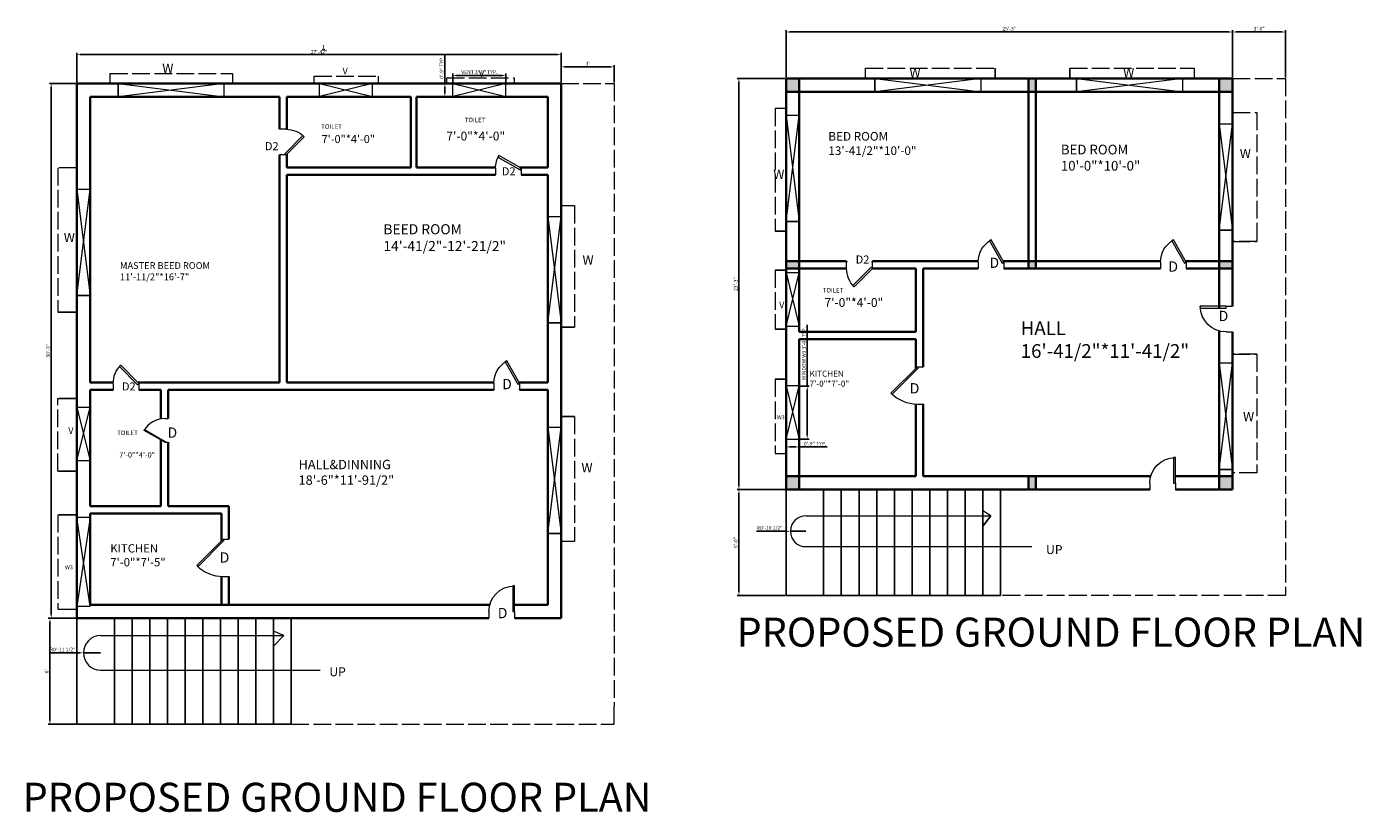
# Model space of a CAD drawing. Units: millimetres. Extents: x 3312 to 4717, y 967 to 1587.
# Tile 2 of 2: x 3811 to 4717, y 1054 to 1587. Entities that reach past the tile are written whole.
import ezdxf

# ---------------------------------------------------------------- set-up
doc = ezdxf.new("R2010")
doc.units = ezdxf.units.MM
doc.linetypes.add('ACAD_ISO02W100', pattern=[15, 12, -3])
for name, color, linetype, lineweight, true_color in [('A-ANNO-DIMS', 116, 'Continuous', 18, 0x136734), ('A-ANNO-IDEN', 116, 'Continuous', 18, 0x136734), ('A-ANNO-SYMB', 219, 'Continuous', 18, 0x642165), ('A-ANNO-TEXT', 55, 'Continuous', 18, 0x999b37), ('A-ANNO-TITL', 116, 'Continuous', 35, 0x136734), ('A-AREA-IDEN', 244, 'Continuous', 18, 0x991b1e), ('A-GLAZ', 219, 'Continuous', 18, 0x642165), ('A-GLAZ-OVHD', 67, 'ACAD_ISO02W100', 13, 0x727430), ('C-PROP', 67, 'ACAD_ISO02W100', 18, 0x727430)]:
    doc.layers.add(name, color=color, linetype=linetype, lineweight=lineweight, true_color=true_color)
for name, color, linetype, lineweight in [('A-COLS', 7, 'Continuous', 35), ('A-COLS-PATT', 7, 'Continuous', 13), ('A-DOOR', 4, 'Continuous', 18), ('A-FLOR-STRS', 7, 'Continuous', 25), ('A-WALL', 7, 'Continuous', 35)]:
    doc.layers.add(name, color=color, linetype=linetype, lineweight=lineweight)
doc.styles.get("Standard").update_dxf_attribs({"font": 'arial.ttf'})
doc.dimstyles.new('ISO-25', dxfattribs={"dimtxt": 2.5, "dimasz": 2.5, "dimexe": 1.25, "dimexo": 0.625, "dimtad": 1, "dimdec": 3, "dimlunit": 4, "dimtxsty": 'Standard', "dimcen": 2.5, "dimadec": 0, "dimazin": 0, "dimtfac": 1, "dimtdec": 3, "dimtmove": 0, "dimatfit": 3, "dimfxl": 1, "dimarcsym": 0})

# ---------------------------------------------------------------- blocks, each defined once
blk = doc.blocks.new('*U2')
for p, q in [((0, 0), (0, -6)), ((24, 0), (24, -6))]:
    blk.add_line(p, q)
blk.add_lwpolyline([(0, 0), (0, 24), (1.75, 24), (1.75, 0)], close=True)
blk.add_arc((0, 0), 24, 0, 90)
blk = doc.blocks.new('*U13')
for p, q in [((0, 0), (0, -6)), ((24, 0), (24, -6))]:
    blk.add_line(p, q)
blk.add_lwpolyline([(0, 0), (12, 20.8), (13.5, 19.9), (1.5, -0.9)], close=True)
blk.add_arc((0, 0), 24, 0, 60)
blk = doc.blocks.new('*U15')
for p, q in [((0, 0), (0, -6)), ((24, 0), (24, -6))]:
    blk.add_line(p, q)
blk.add_lwpolyline([(0, 0), (20.8, 12), (21.7, 10.5), (0.9, -1.5)], close=True)
blk.add_arc((0, 0), 24, 0, 30)
blk = doc.blocks.new('*U6')
for p, q in [((0, 0), (0, 6)), ((40, 0), (40, 6))]:
    blk.add_line(p, q)
blk.add_lwpolyline([(0, 0), (28.3, -28.3), (29.5, -27), (1.2, 1.2)], close=True)
blk.add_arc((0, 0), 40, 315, 360)
blk = doc.blocks.new('*U14')
for p, q in [((0, 0), (0, -6)), ((24, 0), (24, -6))]:
    blk.add_line(p, q)
blk.add_lwpolyline([(0, 0), (17, 17), (18.2, 15.7), (1.2, -1.2)], close=True)
blk.add_arc((0, 0), 24, 0, 45)
blk = doc.blocks.new('*U7')
for p, q in [((0, 0), (0, -6)), ((40, 0), (40, -6))]:
    blk.add_line(p, q)
blk.add_lwpolyline([(0, 0), (20, 34.6), (21.5, 33.8), (1.5, -0.9)], close=True)
blk.add_arc((0, 0), 40, 0, 60)
blk = doc.blocks.new('*D16')
at = {"layer": 'A-ANNO-DIMS', "color": 0, "lineweight": -2, "transparency": 16777216}
for p, q in [((4174.05, 1549.21), (4174.05, 1561.11)), ((4176.55, 1559.86), (4207.55, 1559.86)), ((4210.05, 1549.21), (4210.05, 1561.11))]:
    blk.add_line(p, q, dxfattribs=at)
at = {"layer": 'A-ANNO-DIMS', "color": 0, "lineweight": 5, "transparency": 16777216}
for points in [[(4176.55, 1560.28), (4176.55, 1559.45), (4174.05, 1559.86)], [(4207.55, 1560.28), (4207.55, 1559.45), (4210.05, 1559.86)]]:
    blk.add_solid(points, dxfattribs=at)
at = {"layer": 'Defpoints', "color": 0, "lineweight": 5, "transparency": 16777216}
for p in [(4210.05, 1559.86), (4174.05, 1548.59), (4210.05, 1548.59)]:
    blk.add_point(p, dxfattribs=at)
at = {"layer": 'A-ANNO-DIMS', "color": 0, "transparency": 16777216, "insert": (4192.05, 1561.76), "char_height": 2.5, "attachment_point": 5}
blk.add_mtext("3'", dxfattribs=at)
blk = doc.blocks.new('*D17')
at = {"layer": 'A-ANNO-DIMS', "color": 0, "lineweight": -2, "transparency": 16777216}
for p, q in [((3845.55, 1549.21), (3845.55, 1569.4)), ((4171.55, 1568.15), (3848.05, 1568.15)), ((4174.05, 1549.21), (4174.05, 1569.4))]:
    blk.add_line(p, q, dxfattribs=at)
at = {"layer": 'A-ANNO-DIMS', "color": 0, "lineweight": 5, "transparency": 16777216}
for points in [[(3848.05, 1568.56), (3848.05, 1567.73), (3845.55, 1568.15)], [(4171.55, 1568.56), (4171.55, 1567.73), (4174.05, 1568.15)]]:
    blk.add_solid(points, dxfattribs=at)
at = {"layer": 'Defpoints', "color": 0, "lineweight": 5, "transparency": 16777216}
for p in [(3845.55, 1568.15), (3845.55, 1548.59), (4174.05, 1548.59)]:
    blk.add_point(p, dxfattribs=at)
at = {"layer": 'A-ANNO-DIMS', "color": 0, "transparency": 16777216, "insert": (4009.8, 1571.7), "char_height": 2.5, "attachment_point": 5}
blk.add_mtext('27\'-4{\\H1x;\\S1/2;}"', dxfattribs=at)
blk = doc.blocks.new('*D18')
at = {"layer": 'A-ANNO-DIMS', "color": 0, "lineweight": -2, "transparency": 16777216}
for p, q in [((3844.92, 1548.59), (3826.85, 1548.59)), ((3828.1, 1546.09), (3828.1, 1188.09)), ((3844.92, 1185.59), (3826.85, 1185.59))]:
    blk.add_line(p, q, dxfattribs=at)
at = {"layer": 'A-ANNO-DIMS', "color": 0, "lineweight": 5, "transparency": 16777216}
for points in [[(3827.69, 1546.09), (3828.52, 1546.09), (3828.1, 1548.59)], [(3827.69, 1188.09), (3828.52, 1188.09), (3828.1, 1185.59)]]:
    blk.add_solid(points, dxfattribs=at)
at = {"layer": 'Defpoints', "color": 0, "lineweight": 5, "transparency": 16777216}
for p in [(3845.55, 1548.59), (3828.1, 1185.59), (3845.55, 1185.59)]:
    blk.add_point(p, dxfattribs=at)
at = {"layer": 'A-ANNO-DIMS', "color": 0, "transparency": 16777216, "insert": (3826.2, 1367.09), "char_height": 2.5, "attachment_point": 5, "rotation": 90}
blk.add_mtext('30\'-3"', dxfattribs=at)
blk = doc.blocks.new('*D19')
at = {"layer": 'A-ANNO-DIMS', "color": 0, "lineweight": -2, "transparency": 16777216}
for p, q in [((3844.92, 1185.59), (3825.98, 1185.59)), ((3827.23, 1183.09), (3827.23, 1116.09)), ((3844.92, 1113.59), (3825.98, 1113.59))]:
    blk.add_line(p, q, dxfattribs=at)
at = {"layer": 'A-ANNO-DIMS', "color": 0, "lineweight": 5, "transparency": 16777216}
for points in [[(3826.82, 1183.09), (3827.65, 1183.09), (3827.23, 1185.59)], [(3826.82, 1116.09), (3827.65, 1116.09), (3827.23, 1113.59)]]:
    blk.add_solid(points, dxfattribs=at)
at = {"layer": 'Defpoints', "color": 0, "lineweight": 5, "transparency": 16777216}
for p in [(3845.55, 1185.59), (3827.23, 1113.59), (3845.55, 1113.59)]:
    blk.add_point(p, dxfattribs=at)
at = {"layer": 'A-ANNO-DIMS', "color": 0, "transparency": 16777216, "insert": (3825.33, 1149.59), "char_height": 2.5, "attachment_point": 5, "rotation": 90}
blk.add_mtext("6'", dxfattribs=at)
blk = doc.blocks.new('*U21')
for p, q in [((0, 0), (0, -6)), ((24, 0), (24, -6))]:
    blk.add_line(p, q)
blk.add_lwpolyline([(0, 0), (0, 24), (1.75, 24), (1.75, 0)], close=True)
blk.add_arc((0, 0), 24, 0, 90)
blk = doc.blocks.new('*U20')
for p, q in [((0, 0), (0, 6)), ((24, 0), (24, 6))]:
    blk.add_line(p, q)
blk.add_lwpolyline([(0, 0), (17, -17), (18.2, -15.7), (1.2, 1.2)], close=True)
blk.add_arc((0, 0), 24, 315, 0)
blk = doc.blocks.new('WIN-STANDARD')
for p, q in [((0, 72), (0, 0)), ((0, 0), (9, 72)), ((9, 72), (0, 72)), ((0, 72), (9, 0)), ((9, 0), (9, 72)), ((0, 0), (9, 0)), ((9, 0), (0, 0))]:
    blk.add_line(p, q)
blk = doc.blocks.new('GLAZ-NARROW')
for p, q in [((9, 35.99), (0.01, 35.99)), ((0.01, 35.99), (0.01, 0)), ((0.01, 0), (9, 35.99)), ((0.07, 35.99), (9, 0)), ((9, 0), (9, 35.99)), ((0, 0), (9, 0))]:
    blk.add_line(p, q)
blk = doc.blocks.new('VENT-PLAN')
for p, q in [((36, 9.18), (0, 9.18)), ((36, 9.18), (0, 0.18)), ((0, 0.18), (0, 9.18)), ((0, 9.18), (36, 0.18)), ((36, 0), (36, 9.18)), ((0, 0.18), (36, 0.18))]:
    blk.add_line(p, q)
blk = doc.blocks.new('STAIR-ENTRY-FLIGHT')
for p, q in [((0, 72), (0, 0)), ((145.5, 72), (0, 72)), ((25.5, 0), (25.5, 72)), ((37.5, 0), (37.5, 72)), ((49.5, 0), (49.5, 72)), ((61.5, 0), (61.5, 72)), ((73.5, 0), (73.5, 72)), ((85.5, 0), (85.5, 72)), ((97.5, 0), (97.5, 72)), ((109.5, 0), (109.5, 72)), ((121.5, 0), (121.5, 72)), ((133.5, 0), (133.5, 72)), ((145.5, 0), (145.5, 72)), ((0, 0), (145.5, 0))]:
    blk.add_line(p, q)
blk = doc.blocks.new('*D28')
at = {"layer": 'A-ANNO-DIMS', "color": 0, "lineweight": -2, "transparency": 16777216}
for p, q in [((4341.03, 1343.2), (4341.03, 1384.8)), ((4336.26, 1343.2), (4342.28, 1343.2)), ((4341.03, 1309.72), (4341.03, 1340.7)), ((4336.26, 1307.22), (4342.28, 1307.22))]:
    blk.add_line(p, q, dxfattribs=at)
at = {"layer": 'A-ANNO-DIMS', "color": 0, "lineweight": 5, "transparency": 16777216}
for points in [[(4340.61, 1340.7), (4341.45, 1340.7), (4341.03, 1343.2)], [(4340.61, 1309.72), (4341.45, 1309.72), (4341.03, 1307.22)]]:
    blk.add_solid(points, dxfattribs=at)
at = {"layer": 'Defpoints', "color": 0, "lineweight": 5, "transparency": 16777216}
for p in [(4335.63, 1343.2), (4341.03, 1343.2), (4335.63, 1307.22)]:
    blk.add_point(p, dxfattribs=at)
at = {"layer": 'A-ANNO-DIMS', "color": 0, "transparency": 16777216, "insert": (4339.11, 1365.25), "char_height": 2.5, "attachment_point": 5, "rotation": 90}
blk.add_mtext('WINDOW W3 3\'-0" TYP.', dxfattribs=at)
blk = doc.blocks.new('*D29')
at = {"layer": 'A-ANNO-DIMS', "color": 0, "lineweight": -2, "transparency": 16777216}
for p, q in [((4326.63, 1306.59), (4326.63, 1300.57)), ((4335.63, 1306.59), (4335.63, 1300.57)), ((4329.13, 1301.82), (4333.13, 1301.82)), ((4335.63, 1301.82), (4354.62, 1301.82))]:
    blk.add_line(p, q, dxfattribs=at)
at = {"layer": 'A-ANNO-DIMS', "color": 0, "lineweight": 5, "transparency": 16777216}
for points in [[(4329.13, 1302.24), (4329.13, 1301.4), (4326.63, 1301.82)], [(4333.13, 1302.24), (4333.13, 1301.4), (4335.63, 1301.82)]]:
    blk.add_solid(points, dxfattribs=at)
at = {"layer": 'Defpoints', "color": 0, "lineweight": 5, "transparency": 16777216}
for p in [(4326.63, 1307.22), (4335.63, 1307.22), (4335.63, 1301.82)]:
    blk.add_point(p, dxfattribs=at)
at = {"layer": 'A-ANNO-DIMS', "color": 0, "transparency": 16777216, "insert": (4346.38, 1303.72), "char_height": 2.5, "attachment_point": 5}
blk.add_mtext('0\'-9" TYP.', dxfattribs=at)
blk = doc.blocks.new('*D30')
at = {"layer": 'A-ANNO-DIMS', "color": 0, "lineweight": -2, "transparency": 16777216}
for p, q in [((4100.58, 1549.24), (4100.58, 1555.27)), ((4103.08, 1554.02), (4134.08, 1554.02)), ((4136.58, 1549.24), (4136.58, 1555.27))]:
    blk.add_line(p, q, dxfattribs=at)
at = {"layer": 'A-ANNO-DIMS', "color": 0, "lineweight": 5, "transparency": 16777216}
for points in [[(4103.08, 1554.44), (4103.08, 1553.6), (4100.58, 1554.02)], [(4134.08, 1554.44), (4134.08, 1553.6), (4136.58, 1554.02)]]:
    blk.add_solid(points, dxfattribs=at)
at = {"layer": 'Defpoints', "color": 0, "lineweight": 5, "transparency": 16777216}
for p in [(4100.58, 1548.62), (4136.58, 1554.02), (4136.58, 1548.62)]:
    blk.add_point(p, dxfattribs=at)
at = {"layer": 'A-ANNO-DIMS', "color": 0, "transparency": 16777216, "insert": (4118.58, 1555.92), "char_height": 2.5, "attachment_point": 5}
blk.add_mtext('VENT 3\'-0" TYP.', dxfattribs=at)
blk = doc.blocks.new('*D31')
at = {"layer": 'A-ANNO-DIMS', "color": 0, "lineweight": -2, "transparency": 16777216}
for p, q in [((4095.18, 1548.62), (4095.18, 1567.61)), ((4099.95, 1548.62), (4093.93, 1548.62)), ((4099.95, 1539.44), (4093.93, 1539.44)), ((4095.18, 1541.94), (4095.18, 1546.12))]:
    blk.add_line(p, q, dxfattribs=at)
at = {"layer": 'A-ANNO-DIMS', "color": 0, "lineweight": 5, "transparency": 16777216}
for points in [[(4094.76, 1546.12), (4095.59, 1546.12), (4095.18, 1548.62)], [(4094.76, 1541.94), (4095.59, 1541.94), (4095.18, 1539.44)]]:
    blk.add_solid(points, dxfattribs=at)
at = {"layer": 'Defpoints', "color": 0, "lineweight": 5, "transparency": 16777216}
for p in [(4095.18, 1548.62), (4100.58, 1548.62), (4100.58, 1539.44)]:
    blk.add_point(p, dxfattribs=at)
at = {"layer": 'A-ANNO-DIMS', "color": 0, "transparency": 16777216, "insert": (4093.28, 1559.36), "char_height": 2.5, "attachment_point": 5, "rotation": 90}
blk.add_mtext('0\'-9" TYP.', dxfattribs=at)
blk = doc.blocks.new('*D34')
at = {"layer": 'A-ANNO-DIMS', "color": 0, "lineweight": -2, "transparency": 16777216}
for p, q in [((4326.64, 1552.54), (4326.64, 1584.77)), ((4629.64, 1552.54), (4629.64, 1584.77)), ((4329.14, 1583.52), (4627.14, 1583.52))]:
    blk.add_line(p, q, dxfattribs=at)
at = {"layer": 'A-ANNO-DIMS', "color": 0, "lineweight": 5, "transparency": 16777216}
for points in [[(4329.14, 1583.94), (4329.14, 1583.1), (4326.64, 1583.52)], [(4627.14, 1583.94), (4627.14, 1583.1), (4629.64, 1583.52)]]:
    blk.add_solid(points, dxfattribs=at)
at = {"layer": 'Defpoints', "color": 0, "lineweight": 5, "transparency": 16777216}
for p in [(4629.64, 1583.52), (4326.64, 1551.91), (4629.64, 1551.91)]:
    blk.add_point(p, dxfattribs=at)
at = {"layer": 'A-ANNO-DIMS', "color": 0, "transparency": 16777216, "insert": (4478.14, 1585.42), "char_height": 2.5, "attachment_point": 5}
blk.add_mtext('25\'-3"', dxfattribs=at)
blk = doc.blocks.new('*D35')
at = {"layer": 'A-ANNO-DIMS', "color": 0, "lineweight": -2, "transparency": 16777216}
for p, q in [((4629.64, 1552.54), (4629.64, 1584.77)), ((4665.64, 1552.54), (4665.64, 1584.77)), ((4632.14, 1583.52), (4663.14, 1583.52))]:
    blk.add_line(p, q, dxfattribs=at)
at = {"layer": 'A-ANNO-DIMS', "color": 0, "lineweight": 5, "transparency": 16777216}
for points in [[(4632.14, 1583.94), (4632.14, 1583.1), (4629.64, 1583.52)], [(4663.14, 1583.94), (4663.14, 1583.1), (4665.64, 1583.52)]]:
    blk.add_solid(points, dxfattribs=at)
at = {"layer": 'Defpoints', "color": 0, "lineweight": 5, "transparency": 16777216}
for p in [(4665.64, 1583.52), (4629.64, 1551.91), (4665.64, 1551.91)]:
    blk.add_point(p, dxfattribs=at)
at = {"layer": 'A-ANNO-DIMS', "color": 0, "transparency": 16777216, "insert": (4647.64, 1585.42), "char_height": 2.5, "attachment_point": 5}
blk.add_mtext('3\'-0"', dxfattribs=at)
blk = doc.blocks.new('*D36')
at = {"layer": 'A-ANNO-DIMS', "color": 0, "lineweight": -2, "transparency": 16777216}
for p, q in [((4326.01, 1551.91), (4293.48, 1551.91)), ((4294.73, 1549.41), (4294.73, 1275.41)), ((4326.01, 1272.91), (4293.48, 1272.91))]:
    blk.add_line(p, q, dxfattribs=at)
at = {"layer": 'A-ANNO-DIMS', "color": 0, "lineweight": 5, "transparency": 16777216}
for points in [[(4294.31, 1549.41), (4295.14, 1549.41), (4294.73, 1551.91)], [(4294.31, 1275.41), (4295.14, 1275.41), (4294.73, 1272.91)]]:
    blk.add_solid(points, dxfattribs=at)
at = {"layer": 'Defpoints', "color": 0, "lineweight": 5, "transparency": 16777216}
for p in [(4326.64, 1551.91), (4294.73, 1272.91), (4326.64, 1272.91)]:
    blk.add_point(p, dxfattribs=at)
at = {"layer": 'A-ANNO-DIMS', "color": 0, "transparency": 16777216, "insert": (4292.82, 1412.41), "char_height": 2.5, "attachment_point": 5, "rotation": 90}
blk.add_mtext('23\'-3"', dxfattribs=at)
blk = doc.blocks.new('*D37')
at = {"layer": 'A-ANNO-DIMS', "color": 0, "lineweight": -2, "transparency": 16777216}
for p, q in [((4326.01, 1272.91), (4293.48, 1272.91)), ((4294.73, 1270.41), (4294.73, 1203.44)), ((4326.05, 1200.94), (4293.48, 1200.94))]:
    blk.add_line(p, q, dxfattribs=at)
at = {"layer": 'A-ANNO-DIMS', "color": 0, "lineweight": 5, "transparency": 16777216}
for points in [[(4294.31, 1270.41), (4295.14, 1270.41), (4294.73, 1272.91)], [(4294.31, 1203.44), (4295.14, 1203.44), (4294.73, 1200.94)]]:
    blk.add_solid(points, dxfattribs=at)
at = {"layer": 'Defpoints', "color": 0, "lineweight": 5, "transparency": 16777216}
for p in [(4326.64, 1272.91), (4294.73, 1200.94), (4326.67, 1200.94)]:
    blk.add_point(p, dxfattribs=at)
at = {"layer": 'A-ANNO-DIMS', "color": 0, "transparency": 16777216, "insert": (4292.83, 1236.93), "char_height": 2.5, "attachment_point": 5, "rotation": 90}
blk.add_mtext('6\'-0"', dxfattribs=at)
blk = doc.blocks.new('*D39')
at = {"layer": 'A-ANNO-DIMS', "color": 0, "lineweight": -2, "transparency": 16777216}
for p, q in [((3826.88, 1162.06), (3847.44, 1162.06)), ((3861.62, 1162.06), (3849.94, 1162.06))]:
    blk.add_line(p, q, dxfattribs=at)
at = {"layer": 'A-ANNO-DIMS', "color": 0, "lineweight": 5, "transparency": 16777216}
blk.add_solid([(3847.44, 1162.48), (3847.44, 1161.64), (3849.94, 1162.06)], dxfattribs=at)
at = {"layer": 'Defpoints', "color": 0, "lineweight": 5, "transparency": 16777216}
for p in [(3849.94, 1162.06), (3861.62, 1162.06)]:
    blk.add_point(p, dxfattribs=at)
at = {"layer": 'A-ANNO-DIMS', "color": 0, "transparency": 16777216, "insert": (3835.91, 1163.98), "char_height": 2.5, "attachment_point": 5, "rotation": 359.99985}
blk.add_mtext('R0\'-11 1/2"', dxfattribs=at)
blk = doc.blocks.new('*D40')
at = {"layer": 'A-ANNO-DIMS', "color": 0, "lineweight": -2, "transparency": 16777216}
for p, q in [((4306.55, 1244.61), (4327.1, 1244.61)), ((4340.07, 1244.61), (4329.6, 1244.61))]:
    blk.add_line(p, q, dxfattribs=at)
at = {"layer": 'A-ANNO-DIMS', "color": 0, "lineweight": 5, "transparency": 16777216}
blk.add_solid([(4327.1, 1245.02), (4327.1, 1244.19), (4329.6, 1244.61)], dxfattribs=at)
at = {"layer": 'Defpoints', "color": 0, "lineweight": 5, "transparency": 16777216}
for p in [(4329.6, 1244.61), (4340.07, 1244.61)]:
    blk.add_point(p, dxfattribs=at)
at = {"layer": 'A-ANNO-DIMS', "color": 0, "transparency": 16777216, "insert": (4315.58, 1246.53), "char_height": 2.5, "attachment_point": 5, "rotation": 359.99837}
blk.add_mtext('R0\'-10 1/2"', dxfattribs=at)

msp = doc.modelspace()

# ---------------------------------------------------------------- hatches: boundary and pattern name
at = {"layer": 'A-COLS-PATT'}
h = msp.add_hatch(color=256, dxfattribs=at)
h.dxf.hatch_style = 1
h.paths.add_polyline_path([(4335.6388, 1551.9125), (4326.6388, 1551.9125), (4326.6388, 1542.9125), (4335.6388, 1542.9125)])
h.paths.add_polyline_path([(4496.1388, 1551.9125), (4491.1388, 1551.9125), (4491.1388, 1542.9125), (4496.1388, 1542.9125)])
h.paths.add_polyline_path([(4629.6388, 1551.9125), (4620.6388, 1551.9125), (4620.6388, 1542.9125), (4629.6388, 1542.9125)])
h.paths.add_polyline_path([(4629.6388, 1427.9125), (4620.6388, 1427.9125), (4620.6388, 1422.9125), (4629.6388, 1422.9125)])
h.paths.add_polyline_path([(4496.1388, 1427.9125), (4491.1388, 1427.9125), (4491.1388, 1422.9125), (4496.1388, 1422.9125)])
h.paths.add_polyline_path([(4335.6388, 1427.9125), (4326.6388, 1427.9125), (4326.6388, 1422.9125), (4335.6388, 1422.9125)])
h.paths.add_polyline_path([(4335.6388, 1281.9125), (4326.6388, 1281.9125), (4326.6388, 1272.9125), (4335.6388, 1272.9125)])
h.paths.add_polyline_path([(4496.1388, 1281.9125), (4491.1388, 1281.9125), (4491.1388, 1272.9125), (4496.1388, 1272.9125)])
h.paths.add_polyline_path([(4629.6388, 1281.9125), (4620.6388, 1281.9125), (4620.6388, 1272.9125), (4629.6388, 1272.9125)])

# ---------------------------------------------------------------- linework, layer by layer
at = {"layer": 'A-ANNO-SYMB'}
for p, q in [((4340.0683, 1255.0702), (4465.5395, 1255.0702)), ((4465.5395, 1255.0702), (4460.1704, 1258.5039)), ((4460.1704, 1258.5039), (4460.1704, 1247.968)), ((4465.5395, 1255.0702), (4460.1704, 1247.968)), ((4460.1704, 1247.968), (4465.5395, 1255.0702)), ((4339.59, 1234.1432), (4493.4198, 1234.1432)), ((3861.6187, 1173.7434), (3985.8367, 1173.7434)), ((3985.8367, 1173.7434), (3978.9924, 1176.8647)), ((3978.9924, 1176.8647), (3978.9924, 1166.5937)), ((3985.8367, 1173.7434), (3978.9924, 1166.5937)), ((3978.9924, 1166.5937), (3985.8367, 1173.7434)), ((3861.6187, 1150.3765), (4010.5281, 1150.3765))]:
    msp.add_line(p, q, dxfattribs=at)
for centre, radius in [((4340.0683, 1244.6067), 10.4635), ((3861.6187, 1162.06), 11.6835)]:
    msp.add_arc(centre, radius, 90, 270, dxfattribs=at)
at = {"layer": 'A-COLS'}
for p, q in [((4335.6388, 1551.9125), (4326.6388, 1551.9125)), ((4491.1388, 1551.9125), (4496.1388, 1551.9125)), ((4620.6388, 1551.9125), (4629.6388, 1551.9125)), ((4335.6388, 1542.9125), (4326.6388, 1542.9125)), ((4491.1388, 1542.9125), (4496.1388, 1542.9125)), ((4620.6388, 1542.9125), (4629.6388, 1542.9125)), ((4335.6388, 1427.9125), (4326.6388, 1427.9125)), ((4335.6388, 1422.9125), (4326.6388, 1422.9125)), ((4496.1388, 1422.9125), (4491.1388, 1422.9125)), ((4620.6388, 1427.9125), (4629.6388, 1427.9125)), ((4620.6388, 1422.9125), (4629.6388, 1422.9125)), ((4491.1388, 1272.9125), (4491.1388, 1281.9125)), ((4496.1388, 1272.9125), (4496.1388, 1281.9125))]:
    msp.add_line(p, q, dxfattribs=at)
at = {"layer": 'A-FLOR-STRS'}
for p, q in [((3845.5456, 1185.5855), (3845.4924, 1113.5855)), ((3990.9924, 1185.5855), (3845.5456, 1185.5855)), ((3870.9924, 1113.5855), (3870.9924, 1185.5855)), ((3882.9924, 1113.5855), (3882.9924, 1185.5855)), ((3894.9924, 1113.5855), (3894.9924, 1185.5855)), ((3906.9924, 1113.5855), (3906.9924, 1185.5855)), ((3918.9924, 1113.5855), (3918.9924, 1185.5855)), ((3930.9924, 1113.5855), (3930.9924, 1185.5855)), ((3942.9924, 1113.5855), (3942.9924, 1185.5855)), ((3954.9924, 1113.5855), (3954.9924, 1185.5855)), ((3966.9924, 1113.5855), (3966.9924, 1185.5855)), ((3978.9924, 1113.5855), (3978.9924, 1185.5855)), ((3990.9924, 1113.5855), (3990.9924, 1185.5855)), ((3845.4924, 1113.5855), (3990.9924, 1113.5855))]:
    msp.add_line(p, q, dxfattribs=at)
at = {"layer": 'A-GLAZ'}
for p, q in [((3854.5597, 1253.8313), (3845.5597, 1253.8313)), ((3845.5597, 1253.8313), (3845.5597, 1193.8313)), ((3854.5597, 1253.8313), (3845.5597, 1193.8313)), ((3854.5597, 1193.8313), (3845.5597, 1253.8313)), ((3854.5597, 1193.8313), (3854.5597, 1253.8313)), ((3845.5597, 1193.8313), (3854.5597, 1193.8313))]:
    msp.add_line(p, q, dxfattribs=at)
at = {"layer": 'A-GLAZ-OVHD'}
for p, q in [((4380.5492, 1551.9125), (4380.5492, 1559.0201)), ((4380.5492, 1559.0201), (4468.4423, 1559.0201)), ((4468.4423, 1559.0201), (4468.4423, 1551.9125)), ((4468.4423, 1551.9125), (4468.4423, 1559.0201)), ((4519.1237, 1559.0201), (4519.1237, 1551.9125)), ((4519.1237, 1551.9125), (4519.1237, 1559.0201)), ((4519.1237, 1559.0201), (4603.4799, 1559.0201)), ((4603.4799, 1559.0201), (4603.4799, 1551.9125)), ((3868.1011, 1548.5855), (3868.1011, 1555.4307)), ((3868.1011, 1555.4307), (3951.1078, 1555.4307)), ((3951.1078, 1555.4307), (3951.1078, 1548.5855)), ((4006.4179, 1548.5855), (4006.4179, 1553.6268)), ((4006.4179, 1553.6268), (4049.8985, 1553.6268)), ((4049.8985, 1553.6268), (4049.8985, 1548.5855)), ((4096.4379, 1548.5855), (4096.4379, 1552.3766)), ((4096.4379, 1552.3766), (4142.2842, 1552.3766)), ((4142.2842, 1552.3766), (4142.2842, 1548.5855)), ((4326.6388, 1531.6164), (4319.2266, 1531.6164)), ((4319.2266, 1531.6164), (4319.2266, 1448.4223)), ((3845.5456, 1491.4182), (3832.6593, 1491.4182)), ((3832.6593, 1491.4182), (3832.6593, 1393.4298)), ((4174.0456, 1465.6256), (4183.1025, 1465.6256)), ((4183.1025, 1465.6256), (4183.1025, 1383.2067)), ((4319.2266, 1448.4223), (4326.6388, 1448.4223)), ((4326.6388, 1448.4223), (4319.2266, 1448.4223)), ((4319.2266, 1421.9222), (4326.6388, 1421.9222)), ((4326.6388, 1421.9222), (4319.2266, 1421.9222)), ((4319.2266, 1421.9222), (4319.2266, 1381.8389)), ((3832.6593, 1393.4298), (3845.5456, 1393.4298)), ((3845.5456, 1393.4298), (3832.6593, 1393.4298)), ((4183.1025, 1383.2067), (4174.0456, 1383.2067)), ((4174.0456, 1383.2067), (4183.1025, 1383.2067)), ((4319.2266, 1381.8389), (4326.6388, 1381.8389)), ((4326.6388, 1381.8389), (4319.2266, 1381.8389)), ((4319.2266, 1347.75), (4326.6388, 1347.75)), ((4326.6388, 1347.75), (4319.2266, 1347.75)), ((4319.2266, 1347.75), (4319.2266, 1297.3548)), ((3832.5652, 1285.2796), (3832.6593, 1334.6599)), ((3832.6593, 1334.6599), (3845.5456, 1334.6599)), ((3845.5456, 1334.6599), (3832.6593, 1334.6599)), ((4183.1025, 1322.3994), (4174.0456, 1322.3994)), ((4174.0456, 1322.3994), (4183.1025, 1322.3994)), ((4183.1025, 1322.3994), (4183.1025, 1237.5435)), ((4319.2266, 1297.3548), (4326.6388, 1297.3548)), ((3832.5652, 1285.2796), (3845.5456, 1285.2796)), ((3845.5456, 1285.2796), (3832.5652, 1285.2796)), ((3832.5652, 1255.8087), (3845.5456, 1255.8087)), ((3845.5456, 1255.8087), (3832.5652, 1255.8087)), ((3832.5652, 1255.8087), (3832.5652, 1191.6848)), ((4183.1025, 1237.5435), (4174.0456, 1237.5435)), ((3832.5652, 1191.6848), (3845.5456, 1191.6848))]:
    msp.add_line(p, q, dxfattribs=at)
for points in [[(4629.6388, 1528.9139), (4646.0669, 1528.9139), (4646.0669, 1448.9681), (4646.0669, 1441.312), (4629.6388, 1441.312), (4646.0669, 1441.312)], [(4646.0669, 1364.8047), (4629.6388, 1364.8047), (4646.0669, 1364.8047), (4646.0669, 1284.2042), (4629.6388, 1284.2042)]]:
    msp.add_lwpolyline(points, dxfattribs=at)
at = {"layer": 'A-WALL'}
for p, q in [((3845.5456, 1548.5855), (4174.0456, 1548.5855)), ((3845.5456, 1185.5855), (3845.5456, 1548.5855)), ((4174.0456, 1548.5855), (4174.0456, 1185.5855)), ((4326.6388, 1551.9125), (4629.6388, 1551.9125)), ((4326.6388, 1272.9125), (4326.6388, 1551.9125)), ((4335.6388, 1379.9125), (4335.6388, 1551.9125)), ((4491.1388, 1422.9125), (4491.1388, 1551.9125)), ((4496.1388, 1422.9125), (4496.1388, 1551.9125)), ((4620.6388, 1551.9125), (4620.6388, 1396.1181)), ((4629.6388, 1551.9125), (4629.6388, 1397.3913)), ((3854.5456, 1539.5855), (3983.0456, 1539.5855)), ((3854.5456, 1345.5855), (3854.5456, 1539.5855)), ((3983.0456, 1517.4898), (3983.0456, 1539.5855)), ((3988.0456, 1539.5855), (4072.0456, 1539.5855)), ((3988.0456, 1517.4797), (3988.0456, 1539.5855)), ((4072.0456, 1491.5855), (4072.0456, 1539.5855)), ((4076.0456, 1491.5855), (4076.0456, 1539.5855)), ((4076.0456, 1539.5855), (4165.0456, 1539.5855)), ((4165.0456, 1539.5855), (4165.0456, 1491.5855)), ((4326.6388, 1542.9125), (4629.6388, 1542.9125)), ((3983.0861, 1517.4898), (3983.0456, 1517.4898)), ((3983.0456, 1499.987), (3983.0456, 1500.0286)), ((3983.0456, 1500.0286), (3983.0861, 1500.0286)), ((3983.0456, 1345.5855), (3983.0456, 1499.987)), ((3988.0456, 1491.5855), (3988.0456, 1500.6228)), ((3988.0456, 1491.5855), (4072.0456, 1491.5855)), ((3988.0456, 1486.5855), (4129.5519, 1486.5855)), ((3988.0456, 1345.5855), (3988.0456, 1486.5855)), ((4076.0456, 1491.5855), (4129.5611, 1491.5855)), ((4129.5519, 1486.6539), (4129.5519, 1486.5855)), ((4146.0324, 1491.5855), (4165.0456, 1491.5855)), ((4147.0018, 1486.5855), (4147.0131, 1486.6539)), ((4147.0018, 1486.5855), (4165.0456, 1486.5855)), ((4165.0456, 1486.5855), (4165.0456, 1345.5855)), ((4326.6388, 1427.9125), (4367.7918, 1427.9125)), ((4326.6388, 1422.9125), (4367.7918, 1422.9125)), ((4367.7918, 1427.2778), (4367.7918, 1427.9125)), ((4385.253, 1427.2778), (4385.253, 1427.9125)), ((4385.253, 1427.9125), (4457.0326, 1427.9125)), ((4385.253, 1422.9125), (4414.6388, 1422.9125)), ((4414.6388, 1379.9125), (4414.6388, 1422.9125)), ((4419.6388, 1422.9125), (4457.0208, 1422.9125)), ((4419.6388, 1356.3076), (4419.6388, 1422.9125)), ((4474.1105, 1427.9125), (4580.7462, 1427.9125)), ((4474.482, 1422.9125), (4580.7343, 1422.9125)), ((4597.824, 1427.9125), (4620.6388, 1427.9125)), ((4598.1955, 1422.9125), (4620.6388, 1422.9125)), ((4629.5411, 1397.3913), (4629.6388, 1397.3913)), ((4335.6388, 1379.9125), (4414.6388, 1379.9125)), ((4620.6388, 1380.5298), (4620.6388, 1272.9125)), ((4629.5411, 1379.9301), (4629.6388, 1379.9301)), ((4629.6388, 1379.9301), (4629.6388, 1272.9125)), ((4335.6388, 1272.9125), (4335.6388, 1374.9125)), ((4335.6388, 1374.9125), (4414.6388, 1374.9125)), ((4414.6388, 1355.1876), (4414.6388, 1374.9125)), ((4419.5606, 1356.3076), (4419.6388, 1356.3076)), ((3854.5456, 1345.5855), (3870.1775, 1345.5855)), ((3854.5456, 1340.5855), (3870.1682, 1340.5855)), ((3854.5456, 1261.5855), (3854.5456, 1340.5855)), ((3870.1661, 1340.589), (3870.1682, 1340.5855)), ((3886.9962, 1345.5855), (3983.0456, 1345.5855)), ((3887.6274, 1340.589), (3888.2296, 1340.589)), ((3888.2296, 1340.5855), (3902.5456, 1340.5855)), ((3902.5456, 1320.8442), (3902.5456, 1340.5855)), ((3907.5456, 1340.5855), (4128.432, 1340.5855)), ((3907.5456, 1340.5855), (3983.0456, 1340.5855)), ((3907.5456, 1321.0454), (3907.5456, 1340.5855)), ((3988.0456, 1345.5855), (4128.4388, 1345.5855)), ((4128.432, 1340.7351), (4128.432, 1340.5855)), ((4145.6132, 1345.5855), (4165.0456, 1345.5855)), ((4145.8933, 1340.7351), (4145.8933, 1340.5855)), ((4145.8933, 1340.5855), (4165.0456, 1340.5855)), ((4165.0456, 1340.5855), (4165.0456, 1194.5855)), ((4414.6388, 1281.9125), (4414.6388, 1330.9865)), ((4419.5606, 1330.9617), (4419.6388, 1330.9617)), ((4419.6388, 1281.9125), (4419.6388, 1330.9617)), ((3907.4912, 1321.0454), (3907.5456, 1321.0454)), ((3902.5456, 1261.5855), (3902.5456, 1306.4398)), ((3907.5456, 1304.9634), (3907.4912, 1304.976)), ((3907.5456, 1261.5855), (3907.5456, 1304.9634)), ((4414.6388, 1281.9125), (4326.6388, 1281.9125)), ((4574.0889, 1281.9125), (4419.6388, 1281.9125)), ((4629.6388, 1281.9125), (4590.8872, 1281.9125)), ((4573.426, 1272.9125), (4326.6388, 1272.9125)), ((4629.6388, 1272.9125), (4590.8872, 1272.9125)), ((3854.5456, 1261.5855), (3902.5456, 1261.5855)), ((3907.5456, 1261.5855), (3948.5456, 1261.5855)), ((3948.5456, 1261.5855), (3948.5456, 1256.5855)), ((3854.5456, 1194.5855), (3854.5456, 1256.5855)), ((3854.5456, 1256.5855), (3943.5456, 1256.5855)), ((3943.5456, 1238.0395), (3943.5456, 1256.5855)), ((3948.5456, 1239.2347), (3948.5456, 1256.5855)), ((3948.5427, 1239.2347), (3948.5456, 1239.2347)), ((3943.5456, 1194.5855), (3943.5456, 1213.9171)), ((3948.5456, 1213.8887), (3948.5427, 1213.8889)), ((3948.5456, 1194.5855), (3948.5456, 1213.8887)), ((4125.6209, 1194.5855), (3854.5456, 1194.5855)), ((4125.6209, 1194.5855), (3988.0456, 1194.5855)), ((4165.0456, 1194.5855), (4142.4774, 1194.5855)), ((4125.0161, 1185.5855), (3845.5456, 1185.5855)), ((4125.0161, 1185.6647), (4125.0161, 1185.5855)), ((4142.5042, 1185.5855), (4142.4774, 1185.6647)), ((4174.0456, 1185.5855), (4142.5042, 1185.5855))]:
    msp.add_line(p, q, dxfattribs=at)
at = {"layer": 'C-PROP'}
for p, q in [((4174.0456, 1548.5855), (4210.0456, 1548.5855)), ((4210.0456, 1548.5855), (4210.0456, 1125.8598)), ((4629.6388, 1551.9125), (4665.6388, 1551.9125)), ((4665.6388, 1551.9125), (4665.6388, 1200.9418)), ((4665.6388, 1200.9418), (4472.1704, 1200.9418)), ((4210.0456, 1113.5855), (4210.0456, 1125.8598)), ((3990.9924, 1113.5855), (4210.0456, 1113.5855))]:
    msp.add_line(p, q, dxfattribs=at)

# ---------------------------------------------------------------- block references
at = {"layer": 'A-DOOR'}
for name, p, xscale, yscale, zscale, rotation in [('*U14', (3987.4514, 1500.0286), -0.7275510770565516, 0.7275510770565516, 0.7275510770565516, 270), ('*U21', (4625.1758, 1397.3913), -0.7275510770565516, 0.7275510770565516, 0.7275510770565516, 90), ('*U6', (4415.7587, 1356.3076), 0.6336462587443874, 0.6336462587443874, 0.6336462587443874, 270), ('*U7', (3905.0808, 1304.976), 0.4017342436988492, 0.4017342436988492, 0.4017342436988492, 90), ('*U6', (3944.7408, 1239.2347), 0.6336462587443874, 0.6336462587443874, 0.6336462587443874, 270)]:
    msp.add_blockref(name, p, dxfattribs=dict(at, xscale=xscale, yscale=yscale, zscale=zscale, rotation=rotation))
at = {"layer": 'A-DOOR', "xscale": -0.7275510770565516, "yscale": 0.7275510770565516, "zscale": 0.7275510770565516}
for name, p in [('*U15', (4147.0131, 1491.0192)), ('*U13', (4474.482, 1427.269)), ('*U13', (4598.1955, 1427.269)), ('*U20', (4385.253, 1422.9125)), ('*U13', (4145.8933, 1345.1004)), ('*U14', (3887.6274, 1344.9543)), ('*U2', (4590.8872, 1277.147)), ('*U2', (4142.4774, 1190.03))]:
    msp.add_blockref(name, p, dxfattribs=at)
at = {"layer": 'A-FLOR-STRS'}
msp.add_blockref('STAIR-ENTRY-FLIGHT', (4326.6707, 1200.9421), dxfattribs=at)
at = {"layer": 'A-GLAZ'}
for p, rotation in [((3873.5389, 1548.586), 269.9999999999998), ((4386.9766, 1551.913), 269.9999999999997), ((4523.8019, 1551.913), 269.9999999999998)]:
    msp.add_blockref('WIN-STANDARD', p, dxfattribs=dict(at, rotation=rotation))
for name, p in [('VENT-PLAN', (4010.078, 1539.44)), ('VENT-PLAN', (4100.578, 1539.44)), ('WIN-STANDARD', (4326.6556, 1454.8411)), ('WIN-STANDARD', (4620.4928, 1448.9677)), ('WIN-STANDARD', (3845.5426, 1404.564)), ('WIN-STANDARD', (4165.0426, 1386.07)), ('GLAZ-NARROW', (4326.6314, 1383.9281)), ('WIN-STANDARD', (4620.5219, 1286.6028)), ('GLAZ-NARROW', (4326.6314, 1307.2183)), ('GLAZ-NARROW', (3845.5142, 1292.7306)), ('WIN-STANDARD', (4165.0426, 1242.9802))]:
    msp.add_blockref(name, p, dxfattribs=at)

# ---------------------------------------------------------------- texts
at = {"layer": 'A-ANNO-IDEN', "attachment_point": 1}
for s, width, gutter_width, insert, char_height in [('W', 58.784208, 31.4406, (3903.4742, 1561.9963), 6.2881), ('V', 17.492344, 22.1494, (4025.7937, 1559.2495), 4.4299), ('W', 58.784208, 31.4406, (4410.4091, 1559.0201), 6.2881), ('W', 58.784208, 31.4406, (4555.3743, 1559.0201), 6.2881), ('V', 17.492344, 22.1494, (4118.3266, 1557.2957), 4.4299), ('D2', 38.407199, 27.2994, (3973.1028, 1508.7362), 5.45989), ('W', 58.784208, 31.4406, (4634.5234, 1504.1736), 6.2881), ('D2', 38.407199, 27.2994, (4133.864, 1491.6695), 5.45989), ('W', 58.784208, 31.4406, (4318.0273, 1490.0928), 6.2881), ('W', 58.784208, 31.4406, (3836.6098, 1447.1596), 6.2881), ('W', 58.784208, 31.4406, (4188.567, 1431.896), 6.2881), ('D2', 38.407199, 27.2994, (4373.9423, 1431.8115), 5.45989), ('D', 165.385008, 34.9095, (4464.6797, 1430.3611), 6.9819), ('D', 165.385008, 34.9095, (4586.0844, 1427.7742), 6.9819), ('V', 17.492344, 22.1494, (4322.0125, 1400.4311), 4.4299), ('D', 165.385008, 34.9095, (4620.1623, 1394.2347), 6.9819), ('D2', 38.407199, 27.2994, (3876.114, 1345.624), 5.45989), ('D', 165.385008, 34.9095, (4134.0405, 1347.9939), 6.9819), ('D', 165.385008, 34.9095, (4410.5896, 1345.1365), 6.9819), ('W3', 5.651424, 13.549, (4320.431, 1323.2834), 2.7098), ('W', 58.784208, 31.4406, (4636.7406, 1325.5647), 6.2881), ('V', 17.492344, 22.1494, (3839.6934, 1315.0393), 4.4299), ('D', 165.385008, 34.9095, (3907.0097, 1315.0448), 6.9819), ('W', 58.784208, 31.4406, (4187.8467, 1290.8774), 6.2881), ('D', 165.385008, 34.9095, (3942.4033, 1230.2871), 6.9819), ('W3', 5.651424, 13.549, (3837.4789, 1221.534), 2.7098), ('D', 165.385008, 34.9095, (4131.0664, 1192.5674), 6.9819)]:
    msp.add_mtext_dynamic_manual_height_columns(s, width=width, gutter_width=gutter_width, heights=[0], dxfattribs=dict(at, insert=insert, char_height=char_height))
at = {"layer": 'A-ANNO-TEXT', "char_height": 6.06981, "attachment_point": 1}
for insert in [(4503.053, 1235.2013), (4016.7963, 1152.2241)]:
    msp.add_mtext_dynamic_manual_height_columns('UP', width=66.331887, gutter_width=30.349, heights=[0], dxfattribs=dict(at, insert=insert))
at = {"layer": 'A-ANNO-TITL', "char_height": 19.730766, "attachment_point": 1}
for insert in [(4293.0709, 1185.9627), (3808.7418, 1073.8851)]:
    msp.add_mtext_dynamic_manual_height_columns('PROPOSED GROUND FLOOR PLAN', width=589.074298, gutter_width=98.6538, heights=[0], dxfattribs=dict(at, insert=insert))
at = {"layer": 'A-AREA-IDEN', "attachment_point": 1}
for s, width, gutter_width, insert, char_height in [('TOILET', 58.579718, 15.254, (4108.6614, 1525.3452), 3.0508), ('TOILET', 58.579718, 15.254, (4011.3299, 1520.8655), 3.0508), ('7\'-0"*4\'-0"', 96.905472, 27.1693, (4011.5657, 1513.5545), 5.433863), ('7\'-0"*4\'-0"', 106.788009, 29.9401, (4096.19, 1515.8565), 5.988015), ('BED ROOM\\P13\'-41/2"*10\'-0"', 290.777349, 29.251, (4355.344, 1515.6211), 5.850195), ('BED ROOM\\P10\'-0"*10\'-0"', 258.333822, 32.9127, (4513.1438, 1506.9928), 6.58254), ('BEED ROOM\\P14\'-41/2"-12\'-21/2"', 180.567004, 34.3473, (4053.4907, 1453.058), 6.869451), ('MASTER BEED ROOM\\P11\'-11/2"*16\'-7"', 177.546694, 23, (3874.7289, 1427.2719), 4.600004), ('TOILET', 58.579718, 15.254, (4351.5697, 1409.7274), 3.0508), ('7\'-0"*4\'-0"', 106.788009, 29.9401, (4352.7244, 1402.8572), 5.988015), ('HALL\\P16\'-41/2"*11\'-41/2"', 389.616787, 46.5636, (4485.8575, 1387.1454), 9.312716), ('KITCHEN\\P7\'-0"*7\'-0"', 64.62256, 20.1335, (4342.6467, 1353.5445), 4.0267), ('TOILET', 58.579718, 15.254, (3872.8258, 1312.9105), 3.0508), ('7\'-0"*4\'-0"', 65.162002, 18.2694, (3874.2402, 1298.2533), 3.653884), ('HALL&DINNING\\P18\'-6"*11\'-91/2"', 352.751685, 31.7054, (3995.924, 1293.0641), 6.341079), ('KITCHEN\\P7\'-0"*7\'-5"', 88.481306, 28.1757, (3868.1958, 1235.8159), 5.635139)]:
    msp.add_mtext_dynamic_manual_height_columns(s, width=width, gutter_width=gutter_width, heights=[0], dxfattribs=dict(at, insert=insert, char_height=char_height))

# ---------------------------------------------------------------- dimensions: what is measured, and where the dimension line sits
at = {"layer": 'A-ANNO-DIMS'}
for base, p1, p2, override, picture, middle in [((4629.6388, 1583.5201), (4326.6388, 1551.9125), (4629.6388, 1551.9125), {"dimdec": 1, "dimlfac": 1, "dimrnd": 0, "dimzin": 1, "dimdsep": 46, "dimlunit": 4, "dimfrac": 2}, '*D34', (4478.1388, 1585.4224)), ((4665.6388, 1583.5201), (4629.6388, 1551.9125), (4665.6388, 1551.9125), {"dimdec": 1, "dimlfac": 1, "dimrnd": 0, "dimzin": 1, "dimdsep": 46, "dimlunit": 4, "dimfrac": 2}, '*D35', (4647.6388, 1585.4224)), ((3845.5456, 1568.1464), (4174.0456, 1548.5855), (3845.5456, 1548.5855), {"dimclrd": 0, "dimclre": 0, "dimclrt": 0}, '*D17', (4009.7956, 1571.6983)), ((4210.0456, 1559.8624), (4174.0456, 1548.5855), (4210.0456, 1548.5855), {"dimclrd": 0, "dimclre": 0, "dimclrt": 0}, '*D16', (4192.0456, 1561.7647))]:
    dim = msp.add_linear_dim(base=base, p1=p1, p2=p2, dimstyle='ISO-25', override=override, dxfattribs=at)
    dim.commit()
    dim.dimension.update_dxf_attribs({"geometry": picture, "text_midpoint": middle})
for base, p1, p2, text, picture, middle in [((4095.178, 1548.62), (4100.5779, 1539.4399), (4100.5779, 1548.62), '<> TYP.', '*D31', (4093.2765, 1559.3644)), ((4341.0289, 1343.2034), (4335.6312, 1307.2187), (4335.6312, 1343.2034), 'WINDOW W3 <> TYP.', '*D28', (4339.1095, 1365.2507))]:
    dim = msp.add_linear_dim(base=base, p1=p1, p2=p2, angle=90, text=text, dimstyle='ISO-25', override={"dimdec": 1, "dimlfac": 1, "dimrnd": 0, "dimzin": 1, "dimdsep": 46, "dimlunit": 4, "dimfrac": 2}, dxfattribs=at)
    dim.commit()
    dim.dimension.update_dxf_attribs({"geometry": picture, "text_midpoint": middle})
for base, p1, p2, text, picture, middle in [((4136.5774, 1554.0199), (4100.5779, 1548.62), (4136.5774, 1548.62), 'VENT <> TYP.', '*D30', (4118.5777, 1555.9222)), ((4335.6312, 1301.8209), (4326.6312, 1307.2187), (4335.6312, 1307.2187), '<> TYP.', '*D29', (4346.3755, 1303.7224))]:
    dim = msp.add_linear_dim(base=base, p1=p1, p2=p2, text=text, dimstyle='ISO-25', override={"dimdec": 1, "dimlfac": 1, "dimrnd": 0, "dimzin": 1, "dimdsep": 46, "dimlunit": 4, "dimfrac": 2}, dxfattribs=at)
    dim.commit()
    dim.dimension.update_dxf_attribs({"geometry": picture, "text_midpoint": middle})
for base, p1, p2, override, picture, middle in [((3828.1032, 1185.5855), (3845.5456, 1548.5855), (3845.5456, 1185.5855), {"dimclrd": 0, "dimclre": 0, "dimclrt": 0}, '*D18', (3826.2009, 1367.0855)), ((4294.7266, 1272.9125), (4326.6388, 1551.9125), (4326.6388, 1272.9125), {"dimdec": 1, "dimlfac": 1, "dimrnd": 0, "dimzin": 1, "dimdsep": 46, "dimlunit": 4, "dimfrac": 2}, '*D36', (4292.8243, 1412.4125)), ((4294.7266, 1200.9418), (4326.6388, 1272.9125), (4326.6704, 1200.9418), {"dimdec": 1, "dimlfac": 1, "dimrnd": 0, "dimzin": 1, "dimdsep": 46, "dimlunit": 4, "dimfrac": 2}, '*D37', (4292.8251, 1236.9272)), ((3827.2318, 1113.5855), (3845.5456, 1185.5855), (3845.5456, 1113.5855), {"dimclrd": 0, "dimclre": 0, "dimclrt": 0}, '*D19', (3825.3303, 1149.5855))]:
    dim = msp.add_linear_dim(base=base, p1=p1, p2=p2, angle=90, dimstyle='ISO-25', override=override, dxfattribs=at)
    dim.commit()
    dim.dimension.update_dxf_attribs({"geometry": picture, "text_midpoint": middle})
for center, mpoint, picture, middle in [((4340.0683, 1244.6067), (4329.6048, 1244.607), '*D40', (4315.5769, 1246.525)), ((3861.6187, 1162.06), (3849.9353, 1162.06), '*D39', (3835.9073, 1163.9777))]:
    dim = msp.add_radius_dim(center=center, mpoint=mpoint, dimstyle='ISO-25', override={"dimdec": 1, "dimlfac": 1, "dimrnd": 0, "dimzin": 1, "dimdsep": 46, "dimlunit": 4, "dimfrac": 2}, dxfattribs=at)
    dim.commit()
    dim.dimension.update_dxf_attribs({"geometry": picture, "text_midpoint": middle})

doc.saveas('drawing.dxf')
